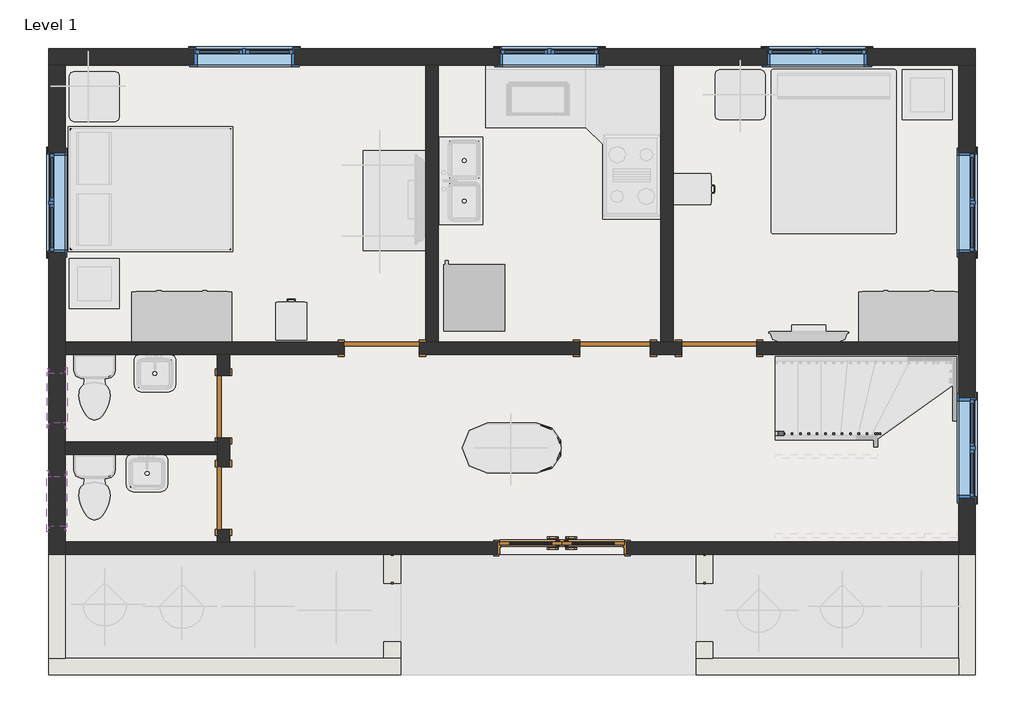
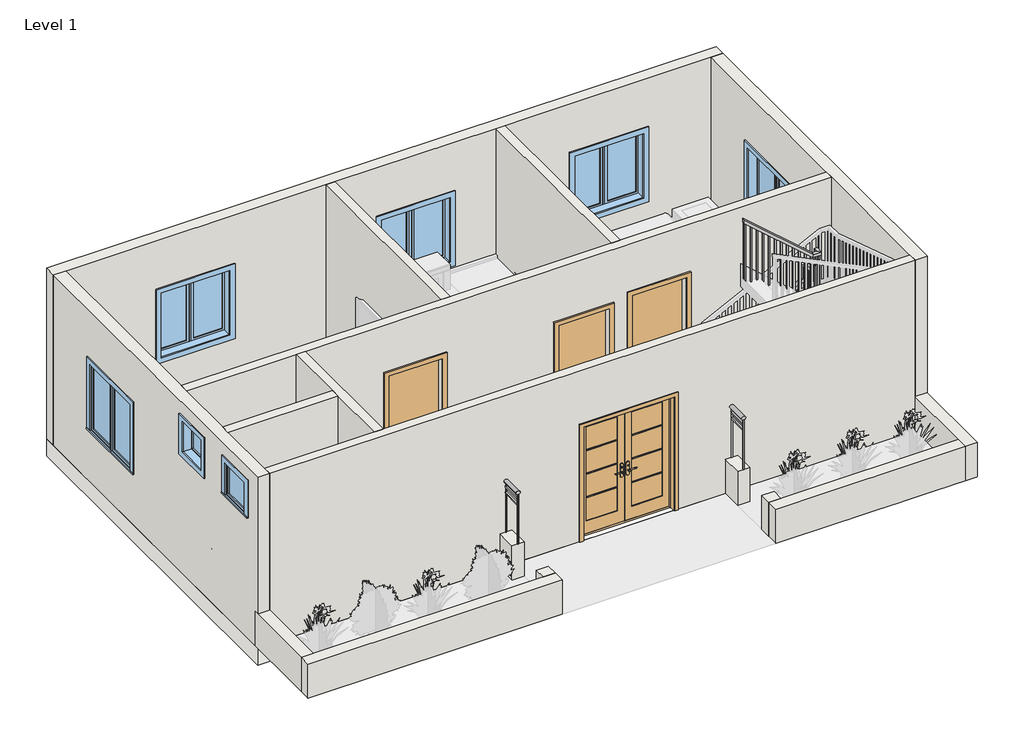
# One storey, part 1 of 2: 17 walls, 8 windows, 6 doors, 3 railings, 1 slab.
"""IFC4 building model written with IfcOpenShell, lengths in millimetres."""

from ifc_helpers import new_model, si_unit, point, frame, origin, origin_with_axes, place, context, project, spatial, polyline, ellipse_curve, trimmed, outline, extrude, faceted_brep, transform, mapped, element, save
from ifc_brep_helpers import plane_surface, extruded_surface, advanced_brep
from components import door_94998e6c, door_255cab33, door_56e8e0a9, door_16372e1c, door_686f89d2, window_0862ab64, window_e41d21a6

model = new_model("IFC4")

# Units and contexts
model_context = context("Model", 3, world=origin())
ifc_project = project(units=[si_unit("LENGTHUNIT", "METRE", prefix="MILLI")], contexts=[model_context])

# Site, building, storey
site = spatial("IfcSite", under=ifc_project)
building = spatial("IfcBuilding", under=site)
storey = spatial("IfcBuildingStorey", under=building, Name="Level 1", Elevation=0.0)

# Doors
placement = place(None, origin())
door_shape = door_94998e6c(model_context)
element("IfcDoor", 1, ObjectType="Door-Exterior-Double-Full Glass-Wood_Clad : 60\" x 80\"", at=placement, inside=storey, context=model_context, shape_type="MappedRepresentation", body=[
    mapped(door_shape, transform((-8050.8118598, 8203.3105643, 0.0), x_axis=(1.0, 0.0, 0.0), y_axis=(0.0, 1.0, 0.0), z_axis=(0.0, 0.0, 1.0))),
])
door_2_shape = door_255cab33(model_context)
element("IfcDoor", 2, ObjectType="Single-Flush : 30\" x 80\"", at=placement, inside=storey, context=model_context, shape_type="MappedRepresentation", body=[
    mapped(door_2_shape, transform((-12178.3118598, 9927.3355643, 0.0), x_axis=(0.0, -1.0, 0.0), y_axis=(1.0, 0.0, 0.0), z_axis=(0.0, 0.0, 1.0))),
])
element("IfcDoor", 3, ObjectType="Single-Flush : 30\" x 80\"", at=placement, inside=storey, context=model_context, shape_type="MappedRepresentation", body=[
    mapped(door_2_shape, transform((-12178.3118598, 8809.7355643, 0.0), x_axis=(0.0, -1.0, 0.0), y_axis=(1.0, 0.0, 0.0), z_axis=(0.0, 0.0, 1.0))),
])
door_3_shape = door_56e8e0a9(model_context)
element("IfcDoor", 4, ObjectType="Single-Flush : 34\" x 80\"", at=placement, inside=storey, context=model_context, shape_type="MappedRepresentation", body=[
    mapped(door_3_shape, transform((-7403.1118598, 10638.5355643, 0.0), x_axis=(1.0, 0.0, 0.0), y_axis=(0.0, 1.0, 0.0), z_axis=(0.0, 0.0, 1.0))),
])
door_4_shape = door_16372e1c(model_context)
element("IfcDoor", 5, ObjectType="Single-Flush : 36\" x 84\"", at=placement, inside=storey, context=model_context, shape_type="MappedRepresentation", body=[
    mapped(door_4_shape, transform((-10247.9118598, 10638.5355643, 0.0), x_axis=(1.0, 0.0, 0.0), y_axis=(0.0, 1.0, 0.0), z_axis=(0.0, 0.0, 1.0))),
])
door_5_shape = door_686f89d2(model_context)
element("IfcDoor", 6, ObjectType="Single-Flush : 36\" x 84\"", at=placement, inside=storey, context=model_context, shape_type="MappedRepresentation", body=[
    mapped(door_5_shape, transform((-6133.1118598, 10638.5355643, 0.0), x_axis=(-1.0, 0.0, 0.0), y_axis=(0.0, -1.0, 0.0), z_axis=(0.0, 0.0, 1.0))),
])

# Railings
element("IfcRailing", 7, ObjectType="Glass Panel - Bottom Fill", at=placement, inside=storey, context=model_context, shape_type="SolidModel", body=[
    advanced_brep(
    [(-10082.8118598, 8123.9355643, 1524.0), (-10159.0118598, 8123.9355643, 1524.0), (-10082.8118598, 7768.3355643, 1524.0), (-10159.0118598, 7768.3355643, 1524.0)],
    [
        (0, 1, ellipse_curve(frame((-10120.9118598, 8123.9355643, 1524.0), z_axis=(0.0, 1.0, 0.0), x_axis=(-1.0, 0.0, 0.0)), 38.1, 28.575)),
        (1, 0, ellipse_curve(frame((-10120.9118598, 8123.9355643, 1524.0), z_axis=(0.0, 1.0, 0.0), x_axis=(-1.0, 0.0, 0.0)), 38.1, 28.575)),
        (2, 3, ellipse_curve(frame((-10120.9118598, 7768.3355643, 1524.0), z_axis=(0.0, -1.0, 0.0), x_axis=(-1.0, 0.0, 0.0)), 38.1, 28.575)),
        (3, 2, ellipse_curve(frame((-10120.9118598, 7768.3355643, 1524.0), z_axis=(0.0, -1.0, 0.0), x_axis=(-1.0, 0.0, 0.0)), 38.1, 28.575)),
        (0, 2),
        (3, 1),
    ],
    [
        plane_surface(frame((-10120.9118598, 8123.9355643, 1524.0), z_axis=(0.0, 1.0, 0.0), x_axis=(0.0, 0.0, -1.0))),
        plane_surface(frame((-10120.9118598, 7768.3355643, 1524.0), z_axis=(0.0, -1.0, 0.0), x_axis=(0.0, 0.0, -1.0))),
        extruded_surface(trimmed(ellipse_curve(frame((-10120.9118598, 7768.3355643, 1524.0), z_axis=(0.0, 1.0, 0.0), x_axis=(-1.0, 0.0, 0.0)), 38.1, 28.575), [point((-10082.8118598, 7768.3355643, 1524.0))], [point((-10159.0118598, 7768.3355643, 1524.0))], True, "CARTESIAN"), (0.0, 355.59999999999945, 0.0), 355.59999999999945),
        extruded_surface(trimmed(ellipse_curve(frame((-10120.9118598, 7768.3355643, 1524.0), z_axis=(0.0, 1.0, 0.0), x_axis=(-1.0, 0.0, 0.0)), 38.1, 28.575), [point((-10159.0118598, 7768.3355643, 1524.0))], [point((-10082.8118598, 7768.3355643, 1524.0))], True, "CARTESIAN"), (0.0, 355.59999999999945, 0.0), 355.59999999999945),
    ],
    [
        (0, [[1, 2]]),
        (1, [[3, 4]]),
        (2, [[-1, 5, -4, 6]]),
        (3, [[-2, -6, -3, -5]]),
    ],
),
    extrude(outline(polyline([(-10133.6118598, 8123.9355643), (-10108.2118598, 8123.9355643), (-10108.2118598, 7768.3355643), (-10133.6118598, 7768.3355643), (-10133.6118598, 8123.9355643)])), frame((0.0, 0.0, 1409.7), z_axis=(0.0, 0.0, 1.0), x_axis=(1.0, 0.0, 0.0)), (0.0, 0.0, 1.0), 25.4),
    extrude(outline(polyline([(-10133.6118598, 8123.9355643), (-10108.2118598, 8123.9355643), (-10108.2118598, 7768.3355643), (-10133.6118598, 7768.3355643), (-10133.6118598, 8123.9355643)])), frame((0.0, 0.0, 1308.1), z_axis=(0.0, 0.0, 1.0), x_axis=(1.0, 0.0, 0.0)), (0.0, 0.0, 1.0), 25.4),
    extrude(outline(polyline([(-10130.4368598, 7781.0355643), (-10111.3868598, 7781.0355643), (-10111.3868598, 7761.9855643), (-10130.4368598, 7761.9855643), (-10130.4368598, 7781.0355643)])), frame((0.0, 0.0, 609.6), z_axis=(0.0, 0.0, 1.0), x_axis=(1.0, 0.0, 0.0)), (0.0, 0.0, 1.0), 885.6788223),
    extrude(outline(polyline([(-10130.4368598, 8130.2855643), (-10111.3868598, 8130.2855643), (-10111.3868598, 8111.2355643), (-10130.4368598, 8111.2355643), (-10130.4368598, 8130.2855643)])), frame((0.0, 0.0, 609.6), z_axis=(0.0, 0.0, 1.0), x_axis=(1.0, 0.0, 0.0)), (0.0, 0.0, 1.0), 885.6788223),
])
element("IfcRailing", 8, ObjectType="Glass Panel - Bottom Fill", at=placement, inside=storey, context=model_context, shape_type="SolidModel", body=[
    advanced_brep(
    [(-6272.8118598, 8123.9355643, 1524.0), (-6349.0118598, 8123.9355643, 1524.0), (-6272.8118598, 7768.3355643, 1524.0), (-6349.0118598, 7768.3355643, 1524.0)],
    [
        (0, 1, ellipse_curve(frame((-6310.9118598, 8123.9355643, 1524.0), z_axis=(0.0, 1.0, 0.0), x_axis=(-1.0, 0.0, 0.0)), 38.1, 28.575)),
        (1, 0, ellipse_curve(frame((-6310.9118598, 8123.9355643, 1524.0), z_axis=(0.0, 1.0, 0.0), x_axis=(-1.0, 0.0, 0.0)), 38.1, 28.575)),
        (2, 3, ellipse_curve(frame((-6310.9118598, 7768.3355643, 1524.0), z_axis=(0.0, -1.0, 0.0), x_axis=(-1.0, 0.0, 0.0)), 38.1, 28.575)),
        (3, 2, ellipse_curve(frame((-6310.9118598, 7768.3355643, 1524.0), z_axis=(0.0, -1.0, 0.0), x_axis=(-1.0, 0.0, 0.0)), 38.1, 28.575)),
        (0, 2),
        (3, 1),
    ],
    [
        plane_surface(frame((-6310.9118598, 8123.9355643, 1524.0), z_axis=(0.0, 1.0, 0.0), x_axis=(0.0, 0.0, -1.0))),
        plane_surface(frame((-6310.9118598, 7768.3355643, 1524.0), z_axis=(0.0, -1.0, 0.0), x_axis=(0.0, 0.0, -1.0))),
        extruded_surface(trimmed(ellipse_curve(frame((-6310.9118598, 7768.3355643, 1524.0), z_axis=(0.0, 1.0, 0.0), x_axis=(-1.0, 0.0, 0.0)), 38.1, 28.575), [point((-6272.8118598, 7768.3355643, 1524.0))], [point((-6349.0118598, 7768.3355643, 1524.0))], True, "CARTESIAN"), (0.0, 355.59999999999945, 0.0), 355.59999999999945),
        extruded_surface(trimmed(ellipse_curve(frame((-6310.9118598, 7768.3355643, 1524.0), z_axis=(0.0, 1.0, 0.0), x_axis=(-1.0, 0.0, 0.0)), 38.1, 28.575), [point((-6349.0118598, 7768.3355643, 1524.0))], [point((-6272.8118598, 7768.3355643, 1524.0))], True, "CARTESIAN"), (0.0, 355.59999999999945, 0.0), 355.59999999999945),
    ],
    [
        (0, [[1, 2]]),
        (1, [[3, 4]]),
        (2, [[-1, 5, -4, 6]]),
        (3, [[-2, -6, -3, -5]]),
    ],
),
    extrude(outline(polyline([(-6323.6118598, 8123.9355643), (-6298.2118598, 8123.9355643), (-6298.2118598, 7768.3355643), (-6323.6118598, 7768.3355643), (-6323.6118598, 8123.9355643)])), frame((0.0, 0.0, 1409.7), z_axis=(0.0, 0.0, 1.0), x_axis=(1.0, 0.0, 0.0)), (0.0, 0.0, 1.0), 25.4),
    extrude(outline(polyline([(-6323.6118598, 8123.9355643), (-6298.2118598, 8123.9355643), (-6298.2118598, 7768.3355643), (-6323.6118598, 7768.3355643), (-6323.6118598, 8123.9355643)])), frame((0.0, 0.0, 1308.1), z_axis=(0.0, 0.0, 1.0), x_axis=(1.0, 0.0, 0.0)), (0.0, 0.0, 1.0), 25.4),
    extrude(outline(polyline([(-6320.4368598, 7781.0355643), (-6301.3868598, 7781.0355643), (-6301.3868598, 7761.9855643), (-6320.4368598, 7761.9855643), (-6320.4368598, 7781.0355643)])), frame((0.0, 0.0, 609.6), z_axis=(0.0, 0.0, 1.0), x_axis=(1.0, 0.0, 0.0)), (0.0, 0.0, 1.0), 885.6788223),
    extrude(outline(polyline([(-6320.4368598, 8130.2855643), (-6301.3868598, 8130.2855643), (-6301.3868598, 8111.2355643), (-6320.4368598, 8111.2355643), (-6320.4368598, 8130.2855643)])), frame((0.0, 0.0, 609.6), z_axis=(0.0, 0.0, 1.0), x_axis=(1.0, 0.0, 0.0)), (0.0, 0.0, 1.0), 885.6788223),
])
element("IfcRailing", 9, ObjectType="Handrail - Rectangular", at=placement, inside=storey, context=model_context, shape_type="SolidModel", body=[
    faceted_brep([(-5447.3118598, 9622.5355643, 1177.683409), (-5447.3118598, 9622.5355643, 1110.1530498), (-5447.3118598, 9571.7355643, 1110.1530498), (-5447.3118598, 9571.7355643, 1177.683409), (-4275.1801679, 9622.5355643, 2204.3121557), (-4224.3801679, 9622.5355643, 2181.2757221), (-4224.3801679, 9571.7355643, 2181.2757221), (-4275.1801679, 9571.7355643, 2204.3121557), (-4275.1801679, 9622.5355643, 2414.6281882), (-4224.3801679, 9622.5355643, 2363.8281882), (-4224.3801679, 9571.7355643, 2363.8281882), (-4275.1801679, 9571.7355643, 2414.6281882), (-4148.1801679, 9622.5355643, 2414.6281882), (-4148.1801679, 9622.5355643, 2363.8281882), (-4198.9801679, 9571.7355643, 2363.8281882), (-4198.9801679, 9571.7355643, 2414.6281882), (-4148.1801679, 9495.5355643, 2414.6281882), (-4148.1801679, 9466.4142305, 2363.8281882), (-4198.9801679, 9466.4142305, 2363.8281882), (-4198.9801679, 9495.5355643, 2414.6281882), (-4148.1801679, 9368.5355643, 2631.5051451), (-4148.1801679, 9317.7355643, 2617.7256424), (-4198.9801679, 9317.7355643, 2617.7256424), (-4198.9801679, 9368.5355643, 2631.5051451), (-4148.1801679, 9368.5355643, 2841.8211776), (-4148.1801679, 9317.7355643, 2791.0211776), (-4198.9801679, 9317.7355643, 2791.0211776), (-4198.9801679, 9368.5355643, 2841.8211776), (-4148.1801679, 9241.5355643, 2841.8211776), (-4148.1801679, 9241.5355643, 2791.0211776), (-4198.9801679, 9292.3355643, 2791.0211776), (-4198.9801679, 9292.3355643, 2841.8211776), (-4275.1801679, 9241.5355643, 2841.8211776), (-4294.2817023, 9241.5355643, 2791.0211776), (-4294.2817023, 9292.3355643, 2791.0211776), (-4275.1801679, 9292.3355643, 2841.8211776), (-5447.3118598, 9241.5355643, 3868.4499243), (-5447.3118598, 9292.3355643, 3868.4499243), (-5447.3118598, 9292.3355643, 3800.9195651), (-5447.3118598, 9241.5355643, 3800.9195651)], [[[0, 1, 2, 3]], [[1, 0, 4, 5]], [[2, 1, 5, 6]], [[3, 2, 6, 7]], [[0, 3, 7, 4]], [[5, 4, 8, 9]], [[6, 5, 9, 10]], [[7, 6, 10, 11]], [[4, 7, 11, 8]], [[9, 8, 12, 13]], [[10, 9, 13, 14]], [[11, 10, 14, 15]], [[8, 11, 15, 12]], [[13, 12, 16, 17]], [[14, 13, 17, 18]], [[15, 14, 18, 19]], [[12, 15, 19, 16]], [[17, 16, 20, 21]], [[18, 17, 21, 22]], [[19, 18, 22, 23]], [[16, 19, 23, 20]], [[21, 20, 24, 25]], [[22, 21, 25, 26]], [[23, 22, 26, 27]], [[20, 23, 27, 24]], [[25, 24, 28, 29]], [[26, 25, 29, 30]], [[27, 26, 30, 31]], [[24, 27, 31, 28]], [[29, 28, 32, 33]], [[30, 29, 33, 34]], [[31, 30, 34, 35]], [[28, 31, 35, 32]], [[36, 37, 38, 39]], [[33, 32, 36, 39]], [[34, 33, 39, 38]], [[35, 34, 38, 37]], [[32, 35, 37, 36]]]),
    extrude(outline(polyline([(3770.9012635, -5413.0390978), (3787.5864856, -5432.0890978), (2709.3333333, -5432.0890978), (2709.3333333, -5413.0390978), (3770.9012635, -5413.0390978)])), frame((0.0, 9257.4105643, 0.0), z_axis=(0.0, 1.0, 0.0), x_axis=(0.0, 0.0, 1.0)), (0.0, 0.0, 1.0), 19.05),
    extrude(outline(polyline([(3681.9134122, -5311.4390978), (3698.5986343, -5330.4890978), (2709.3333333, -5330.4890978), (2709.3333333, -5311.4390978), (3681.9134122, -5311.4390978)])), frame((0.0, 9257.4105643, 0.0), z_axis=(0.0, 1.0, 0.0), x_axis=(0.0, 0.0, 1.0)), (0.0, 0.0, 1.0), 19.05),
    extrude(outline(polyline([(3592.9255609, -5209.8390978), (3609.6107831, -5228.8890978), (2709.3333333, -5228.8890978), (2709.3333333, -5209.8390978), (3592.9255609, -5209.8390978)])), frame((0.0, 9257.4105643, 0.0), z_axis=(0.0, 1.0, 0.0), x_axis=(0.0, 0.0, 1.0)), (0.0, 0.0, 1.0), 19.05),
    extrude(outline(polyline([(3503.9377097, -5108.2390978), (3520.6229318, -5127.2890978), (2540.0, -5127.2890978), (2540.0, -5108.2390978), (3503.9377097, -5108.2390978)])), frame((0.0, 9257.4105643, 0.0), z_axis=(0.0, 1.0, 0.0), x_axis=(0.0, 0.0, 1.0)), (0.0, 0.0, 1.0), 19.05),
    extrude(outline(polyline([(3414.9498584, -5006.6390978), (3431.6350805, -5025.6890978), (2540.0, -5025.6890978), (2540.0, -5006.6390978), (3414.9498584, -5006.6390978)])), frame((0.0, 9257.4105643, 0.0), z_axis=(0.0, 1.0, 0.0), x_axis=(0.0, 0.0, 1.0)), (0.0, 0.0, 1.0), 19.05),
    extrude(outline(polyline([(3325.9620071, -4905.0390978), (3342.6472292, -4924.0890978), (2540.0, -4924.0890978), (2540.0, -4905.0390978), (3325.9620071, -4905.0390978)])), frame((0.0, 9257.4105643, 0.0), z_axis=(0.0, 1.0, 0.0), x_axis=(0.0, 0.0, 1.0)), (0.0, 0.0, 1.0), 19.05),
    extrude(outline(polyline([(3236.9741559, -4803.4390978), (3253.659378, -4822.4890978), (2370.6666667, -4822.4890978), (2370.6666667, -4803.4390978), (3236.9741559, -4803.4390978)])), frame((0.0, 9257.4105643, 0.0), z_axis=(0.0, 1.0, 0.0), x_axis=(0.0, 0.0, 1.0)), (0.0, 0.0, 1.0), 19.05),
    extrude(outline(polyline([(3147.9863046, -4701.8390978), (3164.6715267, -4720.8890978), (2370.6666667, -4720.8890978), (2370.6666667, -4701.8390978), (3147.9863046, -4701.8390978)])), frame((0.0, 9257.4105643, 0.0), z_axis=(0.0, 1.0, 0.0), x_axis=(0.0, 0.0, 1.0)), (0.0, 0.0, 1.0), 19.05),
    extrude(outline(polyline([(3058.9984533, -4600.2390978), (3075.6836754, -4619.2890978), (2201.3333333, -4619.2890978), (2201.3333333, -4600.2390978), (3058.9984533, -4600.2390978)])), frame((0.0, 9257.4105643, 0.0), z_axis=(0.0, 1.0, 0.0), x_axis=(0.0, 0.0, 1.0)), (0.0, 0.0, 1.0), 19.05),
    extrude(outline(polyline([(2970.0106021, -4498.6390978), (2986.6958242, -4517.6890978), (2201.3333333, -4517.6890978), (2201.3333333, -4498.6390978), (2970.0106021, -4498.6390978)])), frame((0.0, 9257.4105643, 0.0), z_axis=(0.0, 1.0, 0.0), x_axis=(0.0, 0.0, 1.0)), (0.0, 0.0, 1.0), 19.05),
    extrude(outline(polyline([(2881.0227508, -4397.0390978), (2897.7079729, -4416.0890978), (2032.0, -4416.0890978), (2032.0, -4397.0390978), (2881.0227508, -4397.0390978)])), frame((0.0, 9257.4105643, 0.0), z_axis=(0.0, 1.0, 0.0), x_axis=(0.0, 0.0, 1.0)), (0.0, 0.0, 1.0), 19.05),
    extrude(outline(polyline([(2792.0348995, -4295.4390978), (2808.7201216, -4314.4890978), (2032.0, -4314.4890978), (2032.0, -4295.4390978), (2792.0348995, -4295.4390978)])), frame((0.0, 9257.4105643, 0.0), z_axis=(0.0, 1.0, 0.0), x_axis=(0.0, 0.0, 1.0)), (0.0, 0.0, 1.0), 19.05),
    extrude(outline(polyline([(9369.1345758, 2529.9519321), (9388.1845758, 2497.4203886), (9388.1845758, 1524.0), (9369.1345758, 1524.0), (9369.1345758, 2529.9519321)])), frame((-4183.1051679, 0.0, 0.0), z_axis=(1.0, 0.0, 0.0), x_axis=(0.0, 1.0, 0.0)), (0.0, 0.0, 1.0), 19.05),
    extrude(outline(polyline([(9470.7345758, 2356.4503666), (9489.7845758, 2323.918823), (9489.7845758, 1524.0), (9470.7345758, 1524.0), (9470.7345758, 2356.4503666)])), frame((-4183.1051679, 0.0, 0.0), z_axis=(1.0, 0.0, 0.0), x_axis=(0.0, 1.0, 0.0)), (0.0, 0.0, 1.0), 19.05),
    extrude(outline(polyline([(2186.3498761, -4218.5868598), (2169.664654, -4237.6368598), (1185.3333333, -4237.6368598), (1185.3333333, -4218.5868598), (2186.3498761, -4218.5868598)])), frame((0.0, 9587.6105643, 0.0), z_axis=(0.0, 1.0, 0.0), x_axis=(0.0, 0.0, 1.0)), (0.0, 0.0, 1.0), 19.05),
    extrude(outline(polyline([(2097.3620248, -4320.1868598), (2080.6768027, -4339.2368598), (1016.0, -4339.2368598), (1016.0, -4320.1868598), (2097.3620248, -4320.1868598)])), frame((0.0, 9587.6105643, 0.0), z_axis=(0.0, 1.0, 0.0), x_axis=(0.0, 0.0, 1.0)), (0.0, 0.0, 1.0), 19.05),
    extrude(outline(polyline([(2008.3741735, -4421.7868598), (1991.6889514, -4440.8368598), (1016.0, -4440.8368598), (1016.0, -4421.7868598), (2008.3741735, -4421.7868598)])), frame((0.0, 9587.6105643, 0.0), z_axis=(0.0, 1.0, 0.0), x_axis=(0.0, 0.0, 1.0)), (0.0, 0.0, 1.0), 19.05),
    extrude(outline(polyline([(1919.3863223, -4523.3868598), (1902.7011001, -4542.4368598), (846.6666667, -4542.4368598), (846.6666667, -4523.3868598), (1919.3863223, -4523.3868598)])), frame((0.0, 9587.6105643, 0.0), z_axis=(0.0, 1.0, 0.0), x_axis=(0.0, 0.0, 1.0)), (0.0, 0.0, 1.0), 19.05),
    extrude(outline(polyline([(1830.398471, -4624.9868598), (1813.7132489, -4644.0368598), (846.6666667, -4644.0368598), (846.6666667, -4624.9868598), (1830.398471, -4624.9868598)])), frame((0.0, 9587.6105643, 0.0), z_axis=(0.0, 1.0, 0.0), x_axis=(0.0, 0.0, 1.0)), (0.0, 0.0, 1.0), 19.05),
    extrude(outline(polyline([(1741.4106197, -4726.5868598), (1724.7253976, -4745.6368598), (677.3333333, -4745.6368598), (677.3333333, -4726.5868598), (1741.4106197, -4726.5868598)])), frame((0.0, 9587.6105643, 0.0), z_axis=(0.0, 1.0, 0.0), x_axis=(0.0, 0.0, 1.0)), (0.0, 0.0, 1.0), 19.05),
    extrude(outline(polyline([(1652.4227684, -4828.1868598), (1635.7375463, -4847.2368598), (677.3333333, -4847.2368598), (677.3333333, -4828.1868598), (1652.4227684, -4828.1868598)])), frame((0.0, 9587.6105643, 0.0), z_axis=(0.0, 1.0, 0.0), x_axis=(0.0, 0.0, 1.0)), (0.0, 0.0, 1.0), 19.05),
    extrude(outline(polyline([(1563.4349172, -4929.7868598), (1546.7496951, -4948.8368598), (508.0, -4948.8368598), (508.0, -4929.7868598), (1563.4349172, -4929.7868598)])), frame((0.0, 9587.6105643, 0.0), z_axis=(0.0, 1.0, 0.0), x_axis=(0.0, 0.0, 1.0)), (0.0, 0.0, 1.0), 19.05),
    extrude(outline(polyline([(1474.4470659, -5031.3868598), (1457.7618438, -5050.4368598), (508.0, -5050.4368598), (508.0, -5031.3868598), (1474.4470659, -5031.3868598)])), frame((0.0, 9587.6105643, 0.0), z_axis=(0.0, 1.0, 0.0), x_axis=(0.0, 0.0, 1.0)), (0.0, 0.0, 1.0), 19.05),
    extrude(outline(polyline([(1385.4592146, -5132.9868598), (1368.7739925, -5152.0368598), (508.0, -5152.0368598), (508.0, -5132.9868598), (1385.4592146, -5132.9868598)])), frame((0.0, 9587.6105643, 0.0), z_axis=(0.0, 1.0, 0.0), x_axis=(0.0, 0.0, 1.0)), (0.0, 0.0, 1.0), 19.05),
    extrude(outline(polyline([(1296.4713634, -5234.5868598), (1279.7861413, -5253.6368598), (338.6666667, -5253.6368598), (338.6666667, -5234.5868598), (1296.4713634, -5234.5868598)])), frame((0.0, 9587.6105643, 0.0), z_axis=(0.0, 1.0, 0.0), x_axis=(0.0, 0.0, 1.0)), (0.0, 0.0, 1.0), 19.05),
    extrude(outline(polyline([(1207.4835121, -5336.1868598), (1190.79829, -5355.2368598), (338.6666667, -5355.2368598), (338.6666667, -5336.1868598), (1207.4835121, -5336.1868598)])), frame((0.0, 9587.6105643, 0.0), z_axis=(0.0, 1.0, 0.0), x_axis=(0.0, 0.0, 1.0)), (0.0, 0.0, 1.0), 19.05),
    extrude(outline(polyline([(-4193.8390978, 9276.4605643), (-4193.8390978, 9257.4105643), (-4212.8890978, 9257.4105643), (-4212.8890978, 9276.4605643), (-4193.8390978, 9276.4605643)])), frame((0.0, 0.0, 1862.6666667), z_axis=(0.0, 0.0, 1.0), x_axis=(1.0, 0.0, 0.0)), (0.0, 0.0, 1.0), 928.354511),
    extrude(outline(polyline([(-4183.1051679, 9276.4605643), (-4164.0551679, 9276.4605643), (-4164.0551679, 9257.4105643), (-4183.1051679, 9257.4105643), (-4183.1051679, 9276.4605643)])), frame((0.0, 0.0, 1862.6666667), z_axis=(0.0, 0.0, 1.0), x_axis=(1.0, 0.0, 0.0)), (0.0, 0.0, 1.0), 928.354511),
    extrude(outline(polyline([(-4183.1051679, 9291.7365529), (-4164.0551679, 9291.7365529), (-4164.0551679, 9272.6865529), (-4183.1051679, 9272.6865529), (-4183.1051679, 9291.7365529)])), frame((0.0, 0.0, 1693.3333333), z_axis=(0.0, 0.0, 1.0), x_axis=(1.0, 0.0, 0.0)), (0.0, 0.0, 1.0), 1097.6878443),
    extrude(outline(polyline([(-4183.1051679, 9591.3845758), (-4164.0551679, 9591.3845758), (-4164.0551679, 9572.3345758), (-4183.1051679, 9572.3345758), (-4183.1051679, 9591.3845758)])), frame((0.0, 0.0, 1354.6666667), z_axis=(0.0, 0.0, 1.0), x_axis=(1.0, 0.0, 0.0)), (0.0, 0.0, 1.0), 1009.1615215),
    extrude(outline(polyline([(-4183.1051679, 9587.6105643), (-4183.1051679, 9606.6605643), (-4164.0551679, 9606.6605643), (-4164.0551679, 9587.6105643), (-4183.1051679, 9587.6105643)])), frame((0.0, 0.0, 1185.3333333), z_axis=(0.0, 0.0, 1.0), x_axis=(1.0, 0.0, 0.0)), (0.0, 0.0, 1.0), 1178.4948549),
    extrude(outline(polyline([(-4212.8890978, 9587.6105643), (-4212.8890978, 9606.6605643), (-4193.8390978, 9606.6605643), (-4193.8390978, 9587.6105643), (-4212.8890978, 9587.6105643)])), frame((0.0, 0.0, 1185.3333333), z_axis=(0.0, 0.0, 1.0), x_axis=(1.0, 0.0, 0.0)), (0.0, 0.0, 1.0), 1178.4948549),
    extrude(outline(polyline([(3784.234343, -5428.2618598), (3800.9195651, -5447.3118598), (2709.3333333, -5447.3118598), (2709.3333333, -5428.2618598), (3784.234343, -5428.2618598)])), frame((0.0, 9257.4105643, 0.0), z_axis=(0.0, 1.0, 0.0), x_axis=(0.0, 0.0, 1.0)), (0.0, 0.0, 1.0), 19.05),
    extrude(outline(polyline([(1126.8382719, -5428.2618598), (1110.1530498, -5447.3118598), (338.6666667, -5447.3118598), (338.6666667, -5428.2618598), (1126.8382719, -5428.2618598)])), frame((0.0, 9587.6105643, 0.0), z_axis=(0.0, 1.0, 0.0), x_axis=(0.0, 0.0, 1.0)), (0.0, 0.0, 1.0), 19.05),
])

# Slab
element("IfcSlab", 10, ObjectType="Generic - 12\"", at=placement, inside=storey, context=model_context, shape_type="SweptSolid", body=[
    extrude(outline(polyline([(-3008.9118598, 14296.1355643), (-3008.9118598, 8123.9355643), (-14311.9118598, 8123.9355643), (-14311.9118598, 14296.1355643), (-3008.9118598, 14296.1355643)])), frame((0.0, 0.0, -304.8), z_axis=(0.0, 0.0, 1.0), x_axis=(1.0, 0.0, 0.0)), (0.0, 0.0, 1.0), 304.8),
])

# Walls
element("IfcWall", 11, ObjectType="Generic - 2'", at=placement, inside=storey, context=model_context, shape_type="Brep", body=[
    faceted_brep([(-3212.1118598, 6853.9355643, 0.0), (-6209.3118598, 6853.9355643, 0.0), (-6412.5118598, 6853.9355643, 0.0), (-6412.5118598, 6853.9355643, 609.6), (-6209.3118598, 6853.9355643, 609.6), (-3212.1118598, 6853.9355643, 609.6), (-3212.1118598, 6650.7355643, 0.0), (-3212.1118598, 6650.7355643, 609.6), (-6412.5118598, 6650.7355643, 609.6), (-6412.5118598, 6650.7355643, 0.0)], [[[0, 1, 2, 3, 4, 5]], [[6, 7, 8, 9]], [[2, 1, 0, 6, 9]], [[5, 4, 3, 8, 7]], [[0, 5, 7, 6]], [[3, 2, 9, 8]]]),
])
element("IfcWall", 12, ObjectType="Generic - 2'", at=placement, inside=storey, context=model_context, shape_type="Brep", body=[
    faceted_brep([(-14108.7118598, 6853.9355643, 0.0), (-14108.7118598, 8123.9355643, 0.0), (-14108.7118598, 8200.1355643, 0.0), (-14108.7118598, 8200.1355643, 609.6), (-14108.7118598, 6853.9355643, 609.6), (-14311.9118598, 6853.9355643, 0.0), (-14311.9118598, 6853.9355643, 609.6), (-14311.9118598, 8200.1355643, 609.6), (-14311.9118598, 8200.1355643, 0.0)], [[[0, 1, 2, 3, 4]], [[5, 6, 7, 8]], [[2, 1, 0, 5, 8]], [[3, 2, 8, 7]], [[4, 3, 7, 6]], [[0, 4, 6, 5]]]),
])
element("IfcWall", 13, ObjectType="Generic - 2'", at=placement, inside=storey, context=model_context, shape_type="SweptSolid", body=[
    extrude(outline(polyline([(-10222.5118598, 7768.3355643), (-10222.5118598, 8123.9355643), (-10019.3118598, 8123.9355643), (-10019.3118598, 7768.3355643), (-10222.5118598, 7768.3355643)])), origin_with_axes(), (0.0, 0.0, 1.0), 609.6),
])
element("IfcWall", 14, ObjectType="Generic - 2'", at=placement, inside=storey, context=model_context, shape_type="SweptSolid", body=[
    extrude(outline(polyline([(-6209.3118598, 7057.1355643), (-6209.3118598, 6853.9355643), (-6412.5118598, 6853.9355643), (-6412.5118598, 7057.1355643), (-6209.3118598, 7057.1355643)])), origin_with_axes(), (0.0, 0.0, 1.0), 609.6),
])
element("IfcWall", 15, ObjectType="Generic - 2'", at=placement, inside=storey, context=model_context, shape_type="Brep", body=[
    faceted_brep([(-3212.1118598, 8200.1355643, 0.0), (-3212.1118598, 8123.9355643, 0.0), (-3212.1118598, 6853.9355643, 0.0), (-3212.1118598, 6650.7355643, 0.0), (-3212.1118598, 6650.7355643, 609.6), (-3212.1118598, 6853.9355643, 609.6), (-3212.1118598, 8200.1355643, 609.6), (-3008.9118598, 8200.1355643, 0.0), (-3008.9118598, 8200.1355643, 609.6), (-3008.9118598, 6650.7355643, 609.6), (-3008.9118598, 6650.7355643, 0.0)], [[[0, 1, 2, 3, 4, 5, 6]], [[7, 8, 9, 10]], [[3, 2, 1, 0, 7, 10]], [[6, 5, 4, 9, 8]], [[0, 6, 8, 7]], [[4, 3, 10, 9]]]),
])
element("IfcWall", 16, ObjectType="Generic - 2'", at=placement, inside=storey, context=model_context, shape_type="Brep", body=[
    faceted_brep([(-10019.3118598, 6853.9355643, 0.0), (-10222.5118598, 6853.9355643, 0.0), (-14108.7118598, 6853.9355643, 0.0), (-14311.9118598, 6853.9355643, 0.0), (-14311.9118598, 6853.9355643, 609.6), (-14108.7118598, 6853.9355643, 609.6), (-10222.5118598, 6853.9355643, 609.6), (-10019.3118598, 6853.9355643, 609.6), (-10019.3118598, 6650.7355643, 0.0), (-10019.3118598, 6650.7355643, 609.6), (-14311.9118598, 6650.7355643, 609.6), (-14311.9118598, 6650.7355643, 0.0)], [[[0, 1, 2, 3, 4, 5, 6, 7]], [[8, 9, 10, 11]], [[3, 2, 1, 0, 8, 11]], [[7, 6, 5, 4, 10, 9]], [[4, 3, 11, 10]], [[0, 7, 9, 8]]]),
])
element("IfcWall", 17, ObjectType="Generic - 2'", at=placement, inside=storey, context=model_context, shape_type="SweptSolid", body=[
    extrude(outline(polyline([(-6209.3118598, 8123.9355643), (-6209.3118598, 7768.3355643), (-6412.5118598, 7768.3355643), (-6412.5118598, 8123.9355643), (-6209.3118598, 8123.9355643)])), origin_with_axes(), (0.0, 0.0, 1.0), 609.6),
])
element("IfcWall", 18, ObjectType="Generic - 2'", at=placement, inside=storey, context=model_context, shape_type="SweptSolid", body=[
    extrude(outline(polyline([(-10222.5118598, 6853.9355643), (-10222.5118598, 7057.1355643), (-10019.3118598, 7057.1355643), (-10019.3118598, 6853.9355643), (-10222.5118598, 6853.9355643)])), origin_with_axes(), (0.0, 0.0, 1.0), 609.6),
])
element("IfcWall", 19, ObjectType="Generic - 8\"", at=placement, inside=storey, context=model_context, shape_type="Brep", body=[
    faceted_brep([(-14311.9118598, 14092.9355643, 0.0), (-14108.7118598, 14092.9355643, 0.0), (-9714.5118598, 14092.9355643, 0.0), (-9562.1118598, 14092.9355643, 0.0), (-6844.3118598, 14092.9355643, 0.0), (-6691.9118598, 14092.9355643, 0.0), (-3212.1118598, 14092.9355643, 0.0), (-3008.9118598, 14092.9355643, 0.0), (-3008.9118598, 14092.9355643, 3048.0), (-3212.1118598, 14092.9355643, 3048.0), (-6691.9118598, 14092.9355643, 3048.0), (-6844.3118598, 14092.9355643, 3048.0), (-9562.1118598, 14092.9355643, 3048.0), (-9714.5118598, 14092.9355643, 3048.0), (-14108.7118598, 14092.9355643, 3048.0), (-14311.9118598, 14092.9355643, 3048.0), (-11314.7118598, 14092.9355643, 2133.6), (-11314.7118598, 14092.9355643, 914.4), (-12533.9118598, 14092.9355643, 914.4), (-12533.9118598, 14092.9355643, 2133.6), (-7593.6118598, 14092.9355643, 2133.6), (-7593.6118598, 14092.9355643, 914.4), (-8812.8118598, 14092.9355643, 914.4), (-8812.8118598, 14092.9355643, 2133.6), (-4329.7118598, 14092.9355643, 2133.6), (-4329.7118598, 14092.9355643, 914.4), (-5548.9118598, 14092.9355643, 914.4), (-5548.9118598, 14092.9355643, 2133.6), (-14311.9118598, 14296.1355643, 0.0), (-14311.9118598, 14296.1355643, 3048.0), (-3008.9118598, 14296.1355643, 3048.0), (-3008.9118598, 14296.1355643, 0.0), (-11314.7118598, 14296.1355643, 2133.6), (-12533.9118598, 14296.1355643, 2133.6), (-12533.9118598, 14296.1355643, 914.4), (-11314.7118598, 14296.1355643, 914.4), (-7593.6118598, 14296.1355643, 2133.6), (-8812.8118598, 14296.1355643, 2133.6), (-8812.8118598, 14296.1355643, 914.4), (-7593.6118598, 14296.1355643, 914.4), (-4329.7118598, 14296.1355643, 2133.6), (-5548.9118598, 14296.1355643, 2133.6), (-5548.9118598, 14296.1355643, 914.4), (-4329.7118598, 14296.1355643, 914.4)], [[[0, 1, 2, 3, 4, 5, 6, 7, 8, 9, 10, 11, 12, 13, 14, 15], [16, 17, 18, 19], [20, 21, 22, 23], [24, 25, 26, 27]], [[28, 29, 30, 31], [32, 33, 34, 35], [36, 37, 38, 39], [40, 41, 42, 43]], [[7, 6, 5, 4, 3, 2, 1, 0, 28, 31]], [[8, 7, 31, 30]], [[0, 15, 29, 28]], [[17, 16, 32, 35]], [[18, 17, 35, 34]], [[19, 18, 34, 33]], [[16, 19, 33, 32]], [[21, 20, 36, 39]], [[22, 21, 39, 38]], [[23, 22, 38, 37]], [[20, 23, 37, 36]], [[25, 24, 40, 43]], [[26, 25, 43, 42]], [[27, 26, 42, 41]], [[24, 27, 41, 40]], [[15, 14, 13, 12, 11, 10, 9, 8, 30, 29]]]),
])
element("IfcWall", 20, ObjectType="Generic - 8\"", at=placement, inside=storey, context=model_context, shape_type="Brep", body=[
    faceted_brep([(-3212.1118598, 14092.9355643, 0.0), (-3212.1118598, 10714.7355643, 0.0), (-3212.1118598, 10562.3355643, 0.0), (-3212.1118598, 8276.3355643, 0.0), (-3212.1118598, 8200.1355643, 0.0), (-3212.1118598, 8200.1355643, 609.6), (-3212.1118598, 8123.9355643, 609.6), (-3212.1118598, 8123.9355643, 3048.0), (-3212.1118598, 8276.3355643, 3048.0), (-3212.1118598, 10562.3355643, 3048.0), (-3212.1118598, 10714.7355643, 3048.0), (-3212.1118598, 14092.9355643, 3048.0), (-3212.1118598, 11806.9355643, 2133.6), (-3212.1118598, 11806.9355643, 914.4), (-3212.1118598, 13026.1355643, 914.4), (-3212.1118598, 13026.1355643, 2133.6), (-3212.1118598, 8809.7355643, 2133.6), (-3212.1118598, 8809.7355643, 914.4), (-3212.1118598, 10028.9355643, 914.4), (-3212.1118598, 10028.9355643, 2133.6), (-3008.9118598, 14092.9355643, 0.0), (-3008.9118598, 14092.9355643, 3048.0), (-3008.9118598, 8123.9355643, 3048.0), (-3008.9118598, 8123.9355643, 609.6), (-3008.9118598, 8200.1355643, 609.6), (-3008.9118598, 8200.1355643, 0.0), (-3008.9118598, 11806.9355643, 2133.6), (-3008.9118598, 13026.1355643, 2133.6), (-3008.9118598, 13026.1355643, 914.4), (-3008.9118598, 11806.9355643, 914.4), (-3008.9118598, 8809.7355643, 2133.6), (-3008.9118598, 10028.9355643, 2133.6), (-3008.9118598, 10028.9355643, 914.4), (-3008.9118598, 8809.7355643, 914.4)], [[[0, 1, 2, 3, 4, 5, 6, 7, 8, 9, 10, 11], [12, 13, 14, 15], [16, 17, 18, 19]], [[20, 21, 22, 23, 24, 25], [26, 27, 28, 29], [30, 31, 32, 33]], [[4, 3, 2, 1, 0, 20, 25]], [[0, 11, 21, 20]], [[5, 4, 25, 24]], [[23, 6, 5, 24]], [[7, 6, 23, 22]], [[13, 12, 26, 29]], [[14, 13, 29, 28]], [[15, 14, 28, 27]], [[12, 15, 27, 26]], [[17, 16, 30, 33]], [[18, 17, 33, 32]], [[19, 18, 32, 31]], [[16, 19, 31, 30]], [[11, 10, 9, 8, 7, 22, 21]]]),
])
element("IfcWall", 21, ObjectType="Generic - 8\"", at=placement, inside=storey, context=model_context, shape_type="Brep", body=[
    faceted_brep([(-14108.7118598, 8200.1355643, 0.0), (-14108.7118598, 8276.3355643, 0.0), (-14108.7118598, 9343.1355643, 0.0), (-14108.7118598, 9495.5355643, 0.0), (-14108.7118598, 10562.3355643, 0.0), (-14108.7118598, 10714.7355643, 0.0), (-14108.7118598, 14092.9355643, 0.0), (-14108.7118598, 14092.9355643, 3048.0), (-14108.7118598, 10714.7355643, 3048.0), (-14108.7118598, 10562.3355643, 3048.0), (-14108.7118598, 9495.5355643, 3048.0), (-14108.7118598, 9343.1355643, 3048.0), (-14108.7118598, 8276.3355643, 3048.0), (-14108.7118598, 8123.9355643, 3048.0), (-14108.7118598, 8123.9355643, 609.6), (-14108.7118598, 8200.1355643, 609.6), (-14108.7118598, 13026.1355643, 2133.6), (-14108.7118598, 13026.1355643, 914.4), (-14108.7118598, 11806.9355643, 914.4), (-14108.7118598, 11806.9355643, 2133.6), (-14108.7118598, 9076.4355643, 2768.6), (-14108.7118598, 9076.4355643, 2159.0), (-14108.7118598, 8466.8355643, 2159.0), (-14108.7118598, 8466.8355643, 2768.6), (-14108.7118598, 9724.1355643, 2768.6), (-14108.7118598, 10333.7355643, 2768.6), (-14108.7118598, 10333.7355643, 2159.0), (-14108.7118598, 9724.1355643, 2159.0), (-14311.9118598, 8200.1355643, 0.0), (-14311.9118598, 8200.1355643, 609.6), (-14311.9118598, 8123.9355643, 609.6), (-14311.9118598, 8123.9355643, 3048.0), (-14311.9118598, 14092.9355643, 3048.0), (-14311.9118598, 14092.9355643, 0.0), (-14311.9118598, 13026.1355643, 2133.6), (-14311.9118598, 11806.9355643, 2133.6), (-14311.9118598, 11806.9355643, 914.4), (-14311.9118598, 13026.1355643, 914.4), (-14311.9118598, 9076.4355643, 2768.6), (-14311.9118598, 8466.8355643, 2768.6), (-14311.9118598, 8466.8355643, 2159.0), (-14311.9118598, 9076.4355643, 2159.0), (-14311.9118598, 9724.1355643, 2768.6), (-14311.9118598, 9724.1355643, 2159.0), (-14311.9118598, 10333.7355643, 2159.0), (-14311.9118598, 10333.7355643, 2768.6)], [[[0, 1, 2, 3, 4, 5, 6, 7, 8, 9, 10, 11, 12, 13, 14, 15], [16, 17, 18, 19], [20, 21, 22, 23], [24, 25, 26, 27]], [[28, 29, 30, 31, 32, 33], [34, 35, 36, 37], [38, 39, 40, 41], [42, 43, 44, 45]], [[6, 5, 4, 3, 2, 1, 0, 28, 33]], [[7, 6, 33, 32]], [[0, 15, 29, 28]], [[14, 30, 29, 15]], [[14, 13, 31, 30]], [[17, 16, 34, 37]], [[18, 17, 37, 36]], [[19, 18, 36, 35]], [[16, 19, 35, 34]], [[21, 20, 38, 41]], [[22, 21, 41, 40]], [[23, 22, 40, 39]], [[20, 23, 39, 38]], [[43, 42, 24, 27]], [[44, 43, 27, 26]], [[45, 44, 26, 25]], [[42, 45, 25, 24]], [[13, 12, 11, 10, 9, 8, 7, 32, 31]]]),
])
element("IfcWall", 22, ObjectType="INNER 6\"", at=placement, inside=storey, context=model_context, shape_type="SweptSolid", body=[
    extrude(outline(polyline([(-9714.5118598, 10714.7355643), (-9714.5118598, 14092.9355643), (-9562.1118598, 14092.9355643), (-9562.1118598, 10714.7355643), (-9714.5118598, 10714.7355643)])), origin_with_axes(), (0.0, 0.0, 1.0), 3048.0),
])
element("IfcWall", 23, ObjectType="INNER 6\"", at=placement, inside=storey, context=model_context, shape_type="Brep", body=[
    faceted_brep([(-6590.3118598, 10714.7355643, 0.0), (-6691.9118598, 10714.7355643, 0.0), (-6844.3118598, 10714.7355643, 0.0), (-6971.3118598, 10714.7355643, 0.0), (-6971.3118598, 10714.7355643, 2032.0), (-7834.9118598, 10714.7355643, 2032.0), (-7834.9118598, 10714.7355643, 0.0), (-9562.1118598, 10714.7355643, 0.0), (-9714.5118598, 10714.7355643, 0.0), (-9790.7118598, 10714.7355643, 0.0), (-9790.7118598, 10714.7355643, 2133.6), (-10705.1118598, 10714.7355643, 2133.6), (-10705.1118598, 10714.7355643, 0.0), (-14108.7118598, 10714.7355643, 0.0), (-14108.7118598, 10714.7355643, 3048.0), (-9714.5118598, 10714.7355643, 3048.0), (-9562.1118598, 10714.7355643, 3048.0), (-6844.3118598, 10714.7355643, 3048.0), (-6691.9118598, 10714.7355643, 3048.0), (-3212.1118598, 10714.7355643, 3048.0), (-3212.1118598, 10714.7355643, 0.0), (-5675.9118598, 10714.7355643, 0.0), (-5675.9118598, 10714.7355643, 2133.6), (-6590.3118598, 10714.7355643, 2133.6), (-6971.3118598, 10562.3355643, 2032.0), (-6971.3118598, 10562.3355643, 0.0), (-6590.3118598, 10562.3355643, 0.0), (-6590.3118598, 10562.3355643, 2133.6), (-5675.9118598, 10562.3355643, 2133.6), (-5675.9118598, 10562.3355643, 0.0), (-3212.1118598, 10562.3355643, 0.0), (-3212.1118598, 10562.3355643, 3048.0), (-12102.1118598, 10562.3355643, 3048.0), (-12254.5118598, 10562.3355643, 3048.0), (-14108.7118598, 10562.3355643, 3048.0), (-14108.7118598, 10562.3355643, 0.0), (-12254.5118598, 10562.3355643, 0.0), (-12102.1118598, 10562.3355643, 0.0), (-10705.1118598, 10562.3355643, 0.0), (-10705.1118598, 10562.3355643, 2133.6), (-9790.7118598, 10562.3355643, 2133.6), (-9790.7118598, 10562.3355643, 0.0), (-7834.9118598, 10562.3355643, 0.0), (-7834.9118598, 10562.3355643, 2032.0)], [[[0, 1, 2, 3, 4, 5, 6, 7, 8, 9, 10, 11, 12, 13, 14, 15, 16, 17, 18, 19, 20, 21, 22, 23]], [[24, 25, 26, 27, 28, 29, 30, 31, 32, 33, 34, 35, 36, 37, 38, 39, 40, 41, 42, 43]], [[38, 37, 36, 35, 13, 12]], [[21, 20, 30, 29]], [[42, 41, 9, 8, 7, 6]], [[26, 25, 3, 2, 1, 0]], [[14, 13, 35, 34]], [[20, 19, 31, 30]], [[10, 9, 41, 40]], [[11, 10, 40, 39]], [[12, 11, 39, 38]], [[27, 26, 0, 23]], [[28, 27, 23, 22]], [[29, 28, 22, 21]], [[4, 3, 25, 24]], [[5, 4, 24, 43]], [[6, 5, 43, 42]], [[19, 18, 17, 16, 15, 14, 34, 33, 32, 31]]]),
])
element("IfcWall", 24, ObjectType="INNER 6\"", at=placement, inside=storey, context=model_context, shape_type="SweptSolid", body=[
    extrude(outline(polyline([(-12254.5118598, 9343.1355643), (-14108.7118598, 9343.1355643), (-14108.7118598, 9495.5355643), (-12254.5118598, 9495.5355643), (-12254.5118598, 9343.1355643)])), origin_with_axes(), (0.0, 0.0, 1.0), 3048.0),
])
element("IfcWall", 25, ObjectType="INNER 6\"", at=placement, inside=storey, context=model_context, shape_type="Brep", body=[
    faceted_brep([(-12102.1118598, 8276.3355643, 0.0), (-12102.1118598, 8428.7355643, 0.0), (-12102.1118598, 8428.7355643, 2032.0), (-12102.1118598, 9190.7355643, 2032.0), (-12102.1118598, 9190.7355643, 0.0), (-12102.1118598, 9546.3355643, 0.0), (-12102.1118598, 9546.3355643, 2032.0), (-12102.1118598, 10308.3355643, 2032.0), (-12102.1118598, 10308.3355643, 0.0), (-12102.1118598, 10562.3355643, 0.0), (-12102.1118598, 10562.3355643, 3048.0), (-12102.1118598, 8276.3355643, 3048.0), (-12254.5118598, 8428.7355643, 2032.0), (-12254.5118598, 8428.7355643, 0.0), (-12254.5118598, 8276.3355643, 0.0), (-12254.5118598, 8276.3355643, 3048.0), (-12254.5118598, 9343.1355643, 3048.0), (-12254.5118598, 9495.5355643, 3048.0), (-12254.5118598, 10562.3355643, 3048.0), (-12254.5118598, 10562.3355643, 0.0), (-12254.5118598, 10308.3355643, 0.0), (-12254.5118598, 10308.3355643, 2032.0), (-12254.5118598, 9546.3355643, 2032.0), (-12254.5118598, 9546.3355643, 0.0), (-12254.5118598, 9495.5355643, 0.0), (-12254.5118598, 9343.1355643, 0.0), (-12254.5118598, 9190.7355643, 0.0), (-12254.5118598, 9190.7355643, 2032.0)], [[[0, 1, 2, 3, 4, 5, 6, 7, 8, 9, 10, 11]], [[12, 13, 14, 15, 16, 17, 18, 19, 20, 21, 22, 23, 24, 25, 26, 27]], [[20, 19, 9, 8]], [[14, 13, 1, 0]], [[26, 25, 24, 23, 5, 4]], [[10, 9, 19, 18]], [[0, 11, 15, 14]], [[6, 5, 23, 22]], [[7, 6, 22, 21]], [[8, 7, 21, 20]], [[2, 1, 13, 12]], [[3, 2, 12, 27]], [[4, 3, 27, 26]], [[11, 10, 18, 17, 16, 15]]]),
])
element("IfcWall", 26, ObjectType="INNER 6\"", at=placement, inside=storey, context=model_context, shape_type="Brep", body=[
    faceted_brep([(-14108.7118598, 8123.9355643, 3048.0), (-14108.7118598, 8123.9355643, 609.6), (-14108.7118598, 8123.9355643, 0.0), (-10222.5118598, 8123.9355643, 0.0), (-10019.3118598, 8123.9355643, 0.0), (-8838.2118598, 8123.9355643, 0.0), (-8838.2118598, 8123.9355643, 2057.4), (-7263.4118598, 8123.9355643, 2057.4), (-7263.4118598, 8123.9355643, 0.0), (-6412.5118598, 8123.9355643, 0.0), (-6209.3118598, 8123.9355643, 0.0), (-3212.1118598, 8123.9355643, 0.0), (-3212.1118598, 8123.9355643, 609.6), (-3212.1118598, 8123.9355643, 3048.0), (-14108.7118598, 8276.3355643, 0.0), (-14108.7118598, 8276.3355643, 3048.0), (-12254.5118598, 8276.3355643, 3048.0), (-12102.1118598, 8276.3355643, 3048.0), (-3212.1118598, 8276.3355643, 3048.0), (-3212.1118598, 8276.3355643, 0.0), (-7263.4118598, 8276.3355643, 0.0), (-7263.4118598, 8276.3355643, 2057.4), (-8838.2118598, 8276.3355643, 2057.4), (-8838.2118598, 8276.3355643, 0.0), (-12102.1118598, 8276.3355643, 0.0), (-12254.5118598, 8276.3355643, 0.0), (-3212.1118598, 8200.1355643, 0.0), (-14108.7118598, 8200.1355643, 0.0)], [[[0, 1, 2, 3, 4, 5, 6, 7, 8, 9, 10, 11, 12, 13]], [[14, 15, 16, 17, 18, 19, 20, 21, 22, 23, 24, 25]], [[19, 26, 11, 10, 9, 8, 20]], [[2, 27, 14, 25, 24, 23, 5, 4, 3]], [[7, 21, 20, 8]], [[21, 7, 6, 22]], [[22, 6, 5, 23]], [[14, 27, 2, 1, 0, 15]], [[11, 26, 19, 18, 13, 12]], [[0, 13, 18, 17, 16, 15]]]),
])
element("IfcWall", 27, ObjectType="INNER 6\"", at=placement, inside=storey, context=model_context, shape_type="SweptSolid", body=[
    extrude(outline(polyline([(-6844.3118598, 10714.7355643), (-6844.3118598, 14092.9355643), (-6691.9118598, 14092.9355643), (-6691.9118598, 10714.7355643), (-6844.3118598, 10714.7355643)])), origin_with_axes(), (0.0, 0.0, 1.0), 3048.0),
])

# Windows
window_shape = window_0862ab64(model_context)
element("IfcWindow", 28, ObjectType="Casement Dbl with Trim : 48\" x 48\"", at=placement, inside=storey, context=model_context, shape_type="MappedRepresentation", body=[
    mapped(window_shape, transform((-11924.3118598, 14175.4855643, 0.0), x_axis=(1.0, 0.0, 0.0), y_axis=(0.0, 1.0, 0.0), z_axis=(0.0, 0.0, 1.0))),
])
element("IfcWindow", 29, ObjectType="Casement Dbl with Trim : 48\" x 48\"", at=placement, inside=storey, context=model_context, shape_type="MappedRepresentation", body=[
    mapped(window_shape, transform((-14191.2618598, 12416.5355643, 0.0), x_axis=(0.0, 1.0, 0.0), y_axis=(-1.0, 0.0, 0.0), z_axis=(0.0, 0.0, 1.0))),
])
element("IfcWindow", 30, ObjectType="Casement Dbl with Trim : 48\" x 48\"", at=placement, inside=storey, context=model_context, shape_type="MappedRepresentation", body=[
    mapped(window_shape, transform((-8203.2118598, 14175.4855643, 0.0), x_axis=(1.0, 0.0, 0.0), y_axis=(0.0, 1.0, 0.0), z_axis=(0.0, 0.0, 1.0))),
])
element("IfcWindow", 31, ObjectType="Casement Dbl with Trim : 48\" x 48\"", at=placement, inside=storey, context=model_context, shape_type="MappedRepresentation", body=[
    mapped(window_shape, transform((-4939.3118598, 14175.4855643, 0.0), x_axis=(1.0, 0.0, 0.0), y_axis=(0.0, 1.0, 0.0), z_axis=(0.0, 0.0, 1.0))),
])
element("IfcWindow", 32, ObjectType="Casement Dbl with Trim : 48\" x 48\"", at=placement, inside=storey, context=model_context, shape_type="MappedRepresentation", body=[
    mapped(window_shape, transform((-3129.5618598, 12416.5355643, 0.0), x_axis=(0.0, -1.0, 0.0), y_axis=(1.0, 0.0, 0.0), z_axis=(0.0, 0.0, 1.0))),
])
element("IfcWindow", 33, ObjectType="Casement Dbl with Trim : 48\" x 48\"", at=placement, inside=storey, context=model_context, shape_type="MappedRepresentation", body=[
    mapped(window_shape, transform((-3129.5618598, 9419.3355643, 0.0), x_axis=(0.0, -1.0, 0.0), y_axis=(1.0, 0.0, 0.0), z_axis=(0.0, 0.0, 1.0))),
])
window_2_shape = window_e41d21a6(model_context)
element("IfcWindow", 34, ObjectType="Transom with Trim : 24\" x 24\"", at=placement, inside=storey, context=model_context, shape_type="MappedRepresentation", body=[
    mapped(window_2_shape, transform((-14210.3118598, 8809.7355643, 0.0), x_axis=(0.0, 1.0, 0.0), y_axis=(-1.0, 0.0, 0.0), z_axis=(0.0, 0.0, 1.0))),
])
element("IfcWindow", 35, ObjectType="Transom with Trim : 24\" x 24\"", at=placement, inside=storey, context=model_context, shape_type="MappedRepresentation", body=[
    mapped(window_2_shape, transform((-14210.3118598, 9990.8355643, 0.0), x_axis=(0.0, -1.0, 0.0), y_axis=(1.0, 0.0, 0.0), z_axis=(0.0, 0.0, 1.0))),
])

save(model, "model.ifc")

# Revit data of these elements
# Type "Door-Exterior-Double-Full Glass-Wood_Clad : 60\" x 80\""
#   Type Mark = "8"
#   Assembly Code = "B2030100"
#   Analytic Construction = "French door, wood frame with double glass"
#   Top Rail = 0' - 4 11/16"
#   Threshold Offset [instance default] = 0' - 0 1/2"
#   Thickness = 0' - 1 3/8"
#   Thermal Resistance (R) = 1.9158 (h·ft²·°F)/BTU
#   Swing Angle [instance default] = 90.00°
#   Stiles = 0' - 4 3/4"
#   Rough Width = 5' - 2"
#   Rough Height = 6' - 9"
#   Panel Width = 2' - 6"
#   Door Offset [instance default] = 0' - 0"
#   Height = 6' - 8"
#   Width = 5' - 0"
#   Heat Transfer Coefficient (U) = 0.5220 BTU/(h·ft²·°F)
#   Bottom Rail = 0' - 9 1/8"
#   Exterior Trim [instance default] = yes
#   Threshold [instance default] = yes
#   Show Grill [instance default] = yes
#   Function = 1
#   Trim Material = Cherry
#   Threshold Material = Cherry
#   Panel Material = Cherry
#   Glazing = Glass
#   Frame Material = Cherry
#   Door Handle Material = Aluminum
#   Visual Light Transmittance = 0
#   Solar Heat Gain Coefficient = 0
#   Wall Closure = (empty or 0)
#   Construction Type = (empty or 0)
# Type "Single-Flush : 30\" x 80\""
#   Type Mark = "5"
#   Construction Type Id = "MDOOR"
#   Assembly Code = "C1020"
#   Analytic Construction = "Metal"
#   Thickness = 0' - 2"
#   Heat Transfer Coefficient (U) = 0.651978 BTU/(h·ft²·°F)
#   Height = 6' - 8"
#   Trim Projection Ext = 0' - 1"
#   Trim Projection Int = 0' - 1"
#   Trim Width = 0' - 3"
#   Width = 2' - 6"
#   Define Thermal Properties by = 1
#   Door Material = Door - Panel
#   Frame Material = Door - Frame
#   Visual Light Transmittance = 0
#   Solar Heat Gain Coefficient = 0
#   Function = (empty or 0)
#   Wall Closure = (empty or 0)
# Type "Single-Flush : 34\" x 80\""
#   Type Mark = "7"
#   Construction Type Id = "MDOOR"
#   Assembly Code = "C1020"
#   Analytic Construction = "Metal"
#   Thickness = 0' - 2"
#   Heat Transfer Coefficient (U) = 0.651978 BTU/(h·ft²·°F)
#   Height = 6' - 8"
#   Trim Projection Ext = 0' - 1"
#   Trim Projection Int = 0' - 1"
#   Trim Width = 0' - 3"
#   Width = 2' - 10"
#   Define Thermal Properties by = 1
#   Door Material = Door - Panel
#   Frame Material = Door - Frame
#   Visual Light Transmittance = 0
#   Solar Heat Gain Coefficient = 0
#   Function = (empty or 0)
#   Wall Closure = (empty or 0)
# Type "Single-Flush : 36\" x 84\""
#   Type Mark = "1"
#   Construction Type Id = "MDOOR"
#   Assembly Code = "C1020"
#   Analytic Construction = "Metal"
#   Thickness = 0' - 2"
#   Heat Transfer Coefficient (U) = 0.651978 BTU/(h·ft²·°F)
#   Height = 7' - 0"
#   Trim Projection Ext = 0' - 1"
#   Trim Projection Int = 0' - 1"
#   Trim Width = 0' - 3"
#   Width = 3' - 0"
#   Define Thermal Properties by = 1
#   Door Material = Door - Panel
#   Frame Material = Door - Frame
#   Visual Light Transmittance = 0
#   Solar Heat Gain Coefficient = 0
#   Function = (empty or 0)
#   Wall Closure = (empty or 0)
# Type "Glass Panel - Bottom Fill"
#   Assembly Code = "C2010400"
#   built-in parameter 1008612 = 0.0416667 (stored number, unit not read)
#   built-in parameter 1008611 = 0.0416667 (stored number, unit not read)
#   built-in parameter 1008609 = 0.333333 (stored number, unit not read)
#   built-in parameter 1008604 = 0.166667 (stored number, unit not read)
#   built-in parameter 1008603 = 0.166667 (stored number, unit not read)
#   Railing Height = 3' - 0"
#   built-in parameter 1008630 = 2
#   built-in parameter 1008610 = 2
#   built-in parameter 1008618 = Baluster - Square : 3/4"
# Type "Handrail - Rectangular"
#   Assembly Code = "C2010400"
#   built-in parameter 1008612 = 0.0416667 (stored number, unit not read)
#   built-in parameter 1008611 = 0.0416667 (stored number, unit not read)
#   built-in parameter 1008609 = 0.333333 (stored number, unit not read)
#   built-in parameter 1008604 = 0.166667 (stored number, unit not read)
#   built-in parameter 1008603 = 0.166667 (stored number, unit not read)
#   Railing Height = 3' - 0"
#   built-in parameter 1008630 = 2
#   built-in parameter 1008610 = 2
#   built-in parameter 1008618 = Baluster - Square : 3/4"
# Type "Generic - 12\""
#   Assembly Code = "B1010"
#   Function = 0
#   Layers, outside or top first: 1' - 0" no material (function 1)
# Type "Generic - 2'"
#   Assembly Code = "B2010"
#   Layers, outside or top first: 0' - 8" "Birch" (function 1)
# Type "Generic - 8\""
#   Assembly Code = "B2010"
#   Layers, outside or top first: 0' - 8" "Brick, Common" (function 1)
# Type "INNER 6\""
#   Assembly Code = "B2010"
#   Layers, outside or top first: 0' - 6" "Brick, Common" (function 1)
# Type "Casement Dbl with Trim : 48\" x 48\""
#   Type Mark = "10"
#   Construction Type Id = "GSP4R"
#   Assembly Code = "B2020100"
#   Analytic Construction = "1/8 in Pilkington single glazing"
#   Visual Light Transmittance = 0.9
#   Solar Heat Gain Coefficient = 0.78
#   Heat Transfer Coefficient (U) = 0.6496 BTU/(h·ft²·°F)
#   Height = 4' - 0"
#   Default Sill Height = 3' - 0"
#   Trim Projection - Ext. = 0' - 0 1/2"
#   Trim Projection - Int. = 0' - 0 3/4"
#   Trim Width - Exterior = 0' - 3 1/2"
#   Trim Width - Interior = 0' - 3 1/2"
#   Width = 4' - 0"
#   Window Inset = 0' - 0 3/4"
#   Define Thermal Properties by = 1
#   Glass Pane Material = Glass
#   Sash Material = Sash
#   Trim Exterior Material = Trim
#   Trim Interior Material = Trim
#   Wall Closure = (empty or 0)
# Type "Transom with Trim : 24\" x 24\""
#   Type Mark = "13"
#   Construction Type Id = "GSP4R"
#   Assembly Code = "B2020100"
#   Analytic Construction = "1/8 in Pilkington single glazing"
#   Visual Light Transmittance = 0.9
#   Solar Heat Gain Coefficient = 0.78
#   Heat Transfer Coefficient (U) = 0.6496 BTU/(h·ft²·°F)
#   Height = 2' - 0"
#   Default Sill Height = 7' - 1"
#   Trim Projection - Ext. = 0' - 0 1/2"
#   Trim Projection - Int. = 0' - 0 3/4"
#   Trim Width - Exterior = 0' - 3 1/2"
#   Trim Width - Interior = 0' - 3 1/2"
#   Width = 2' - 0"
#   Window Inset = 0' - 0 3/4"
#   Define Thermal Properties by = 1
#   Glass Pane Material = Glass
#   Sash Material = Sash
#   Trim Exterior Material = Trim
#   Trim Interior Material = Trim
#   Wall Closure = (empty or 0)
# Element 1 (IfcDoor, "Door-Exterior-Double-Full Glass-Wood_Clad : 60\" x 80\"")
#   Threshold Offset = 0' - 0 1/2"
#   Swing Angle = 90.00°
#   Door Offset = 0' - 0"
#   Threshold = yes
#   Show Grill = yes
#   Exterior Trim = yes
#   Phase Created = New Construction
#   Materials on its faces: "Cherry", "Aluminum", "Glass"
# Elements 2, 3 (IfcDoor, "Single-Flush : 30\" x 80\"")
#   Phase Created = New Construction
#   Materials on its faces: "Door - Frame", "Door - Panel"
# Element 4 (IfcDoor, "Single-Flush : 34\" x 80\"")
#   Phase Created = New Construction
#   Materials on its faces: "Door - Frame", "Door - Panel"
# Elements 5, 6 (IfcDoor, "Single-Flush : 36\" x 84\"")
#   Phase Created = New Construction
#   Materials on its faces: "Door - Frame", "Door - Panel"
# Elements 7, 8 (IfcRailing, "Glass Panel - Bottom Fill")
#   built-in parameter 1008621 = 2 (stored number, unit not read)
#   Phase Created = New Construction
# Element 9 (IfcRailing, "Handrail - Rectangular")
#   Phase Created = New Construction
# Element 10 (IfcSlab, "Generic - 12\"")
#   Height Offset From Level = 0' - 0"
#   Phase Created = New Construction
#   Materials on its faces: "Default Floor"
# Elements 11, 12, 13, 14, 15, 16, 17, 18 (IfcWall, "Generic - 2'")
#   Top Offset = 0' - 0"
#   Base Offset = 0' - 0"
#   Unconnected Height = 2' - 0"
#   wall height = 2' - 0"
#   Phase Created = New Construction
#   Base Constraint = Level 1
#   Materials on its faces: "Birch"
# Elements 19, 20, 21 (IfcWall, "Generic - 8\"")
#   Top Offset = 0' - 0"
#   Base Offset = 0' - 0"
#   Unconnected Height = 10' - 0"
#   wall height = 10' - 0"
#   Phase Created = New Construction
#   Base Constraint = Level 1
#   Materials on its faces: "Brick, Common"
# Elements 22, 23, 24, 25, 26, 27 (IfcWall, "INNER 6\"")
#   Top Offset = 0' - 0"
#   Base Offset = 0' - 0"
#   Unconnected Height = 10' - 0"
#   wall height = 10' - 0"
#   Phase Created = New Construction
#   Base Constraint = Level 1
#   Materials on its faces: "Brick, Common"
# Element 28 (IfcWindow, "Casement Dbl with Trim : 48\" x 48\"")
#   Mark = "1"
#   Phase Created = New Construction
#   Materials on its faces: "Sash", "Trim", "Glass"
# Element 29 (IfcWindow, "Casement Dbl with Trim : 48\" x 48\"")
#   Mark = "2"
#   Phase Created = New Construction
#   Materials on its faces: "Sash", "Trim", "Glass"
# Element 30 (IfcWindow, "Casement Dbl with Trim : 48\" x 48\"")
#   Mark = "3"
#   Phase Created = New Construction
#   Materials on its faces: "Sash", "Trim", "Glass"
# Element 31 (IfcWindow, "Casement Dbl with Trim : 48\" x 48\"")
#   Mark = "4"
#   Phase Created = New Construction
#   Materials on its faces: "Sash", "Trim", "Glass"
# Element 32 (IfcWindow, "Casement Dbl with Trim : 48\" x 48\"")
#   Mark = "5"
#   Phase Created = New Construction
#   Materials on its faces: "Sash", "Trim", "Glass"
